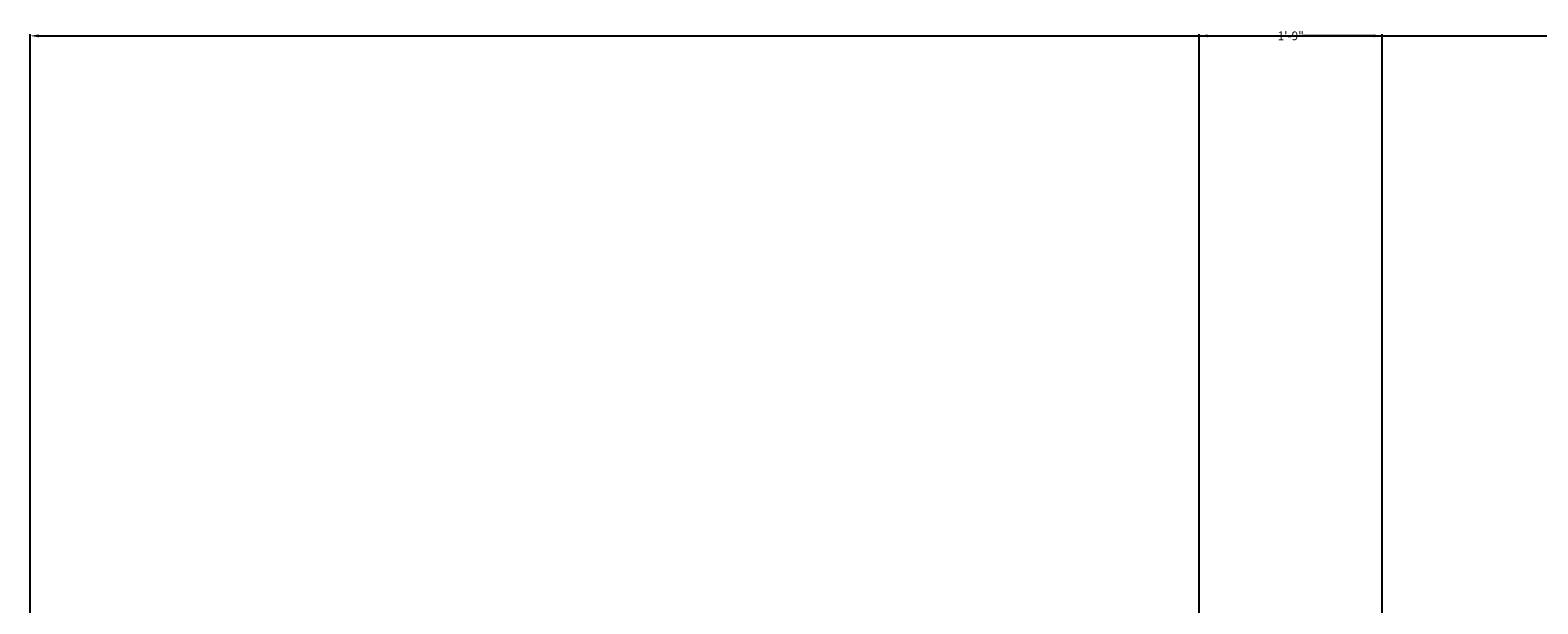
# Model space of a CAD drawing. Units: inches. Extents: x 371 to 1095, y -45 to 1219.
# Tile 17 of 18: x 493 to 666, y 1028 to 1094. Entities that reach past the tile are written whole.
import ezdxf

# ---------------------------------------------------------------- set-up
doc = ezdxf.new("R2010")
doc.units = ezdxf.units.IN
doc.header["$MEASUREMENT"] = 0
doc.layers.add('A-ANNO-DIMS', color=2, linetype='Continuous', lineweight=18)
doc.styles.get("Standard").update_dxf_attribs({"font": 'arial.ttf'})
doc.dimstyles.get("Standard").update_dxf_attribs({"dimtxt": 1, "dimasz": 1, "dimexe": 0.18, "dimexo": 0.0625, "dimgap": 0.09, "dimtad": 0, "dimtih": 1, "dimtoh": 1, "dimdec": 0, "dimzin": 0, "dimdsep": 46, "dimlunit": 3, "dimtxsty": 'Standard', "dimcen": 0.09, "dimadec": 0, "dimazin": 0, "dimtfac": 1, "dimtdec": 0, "dimtofl": 0, "dimtmove": 0, "dimatfit": 3, "dimfxl": 1, "dimtolj": 1, "dimtzin": 0, "dimarcsym": 0})

# ---------------------------------------------------------------- blocks, each defined once
blk = doc.blocks.new('*D50')
at = {"layer": 'A-ANNO-DIMS', "color": 0, "lineweight": -2, "transparency": 16777216}
for p, q in [((492.81, 982.09), (492.81, 1093.41)), ((493.81, 1093.23), (760.98, 1093.23)), ((1031.81, 1093.23), (764.64, 1093.23)), ((1032.81, 982.09), (1032.81, 1093.41))]:
    blk.add_line(p, q, dxfattribs=at)
at = {"layer": 'A-ANNO-DIMS', "color": 0, "transparency": 16777216}
for points in [[(493.81, 1093.39), (493.81, 1093.06), (492.81, 1093.23)], [(1031.81, 1093.39), (1031.81, 1093.06), (1032.81, 1093.23)]]:
    blk.add_solid(points, dxfattribs=at)
at = {"layer": 'Defpoints', "color": 0, "transparency": 16777216}
for p in [(1032.81, 1093.23), (492.81, 982.03), (1032.81, 982.03)]:
    blk.add_point(p, dxfattribs=at)
at = {"layer": 'A-ANNO-DIMS', "color": 0, "transparency": 16777216, "insert": (762.81, 1093.23), "char_height": 1, "attachment_point": 5}
blk.add_mtext('\\A1;45\'-0"', dxfattribs=at)
blk = doc.blocks.new('*D58')
at = {"layer": 'A-ANNO-DIMS', "color": 0, "lineweight": -2, "transparency": 16777216}
for p, q in [((626.74, 973.09), (626.74, 1093.41)), ((627.74, 1093.23), (635.86, 1093.23)), ((646.74, 1093.23), (638.61, 1093.23)), ((647.74, 973.09), (647.74, 1093.41))]:
    blk.add_line(p, q, dxfattribs=at)
at = {"layer": 'A-ANNO-DIMS', "color": 0, "transparency": 16777216}
for points in [[(627.74, 1093.39), (627.74, 1093.06), (626.74, 1093.23)], [(646.74, 1093.39), (646.74, 1093.06), (647.74, 1093.23)]]:
    blk.add_solid(points, dxfattribs=at)
at = {"layer": 'Defpoints', "color": 0, "transparency": 16777216}
for p in [(647.74, 1093.23), (626.74, 973.03), (647.74, 973.03)]:
    blk.add_point(p, dxfattribs=at)
at = {"layer": 'A-ANNO-DIMS', "color": 0, "transparency": 16777216, "insert": (637.24, 1093.23), "char_height": 1, "attachment_point": 5}
blk.add_mtext('\\A1;1\'-9"', dxfattribs=at)

msp = doc.modelspace()

# ---------------------------------------------------------------- dimensions: what is measured, and where the dimension line sits
at = {"layer": 'A-ANNO-DIMS'}
for base, p1, p2, picture, middle in [((1032.81, 1093.23), (492.81, 982.03), (1032.81, 982.03), '*D50', (762.81, 1093.23)), ((647.74, 1093.23), (626.74, 973.03), (647.74, 973.03), '*D58', (637.24, 1093.23))]:
    dim = msp.add_linear_dim(base=base, p1=p1, p2=p2, dimstyle='Standard', override={"dimdec": 1, "dimlfac": 1, "dimrnd": 0, "dimzin": 1, "dimdsep": 46, "dimlunit": 4, "dimfrac": 2}, dxfattribs=at)
    dim.commit()
    dim.dimension.update_dxf_attribs({"geometry": picture, "text_midpoint": middle})

doc.saveas('drawing.dxf')
